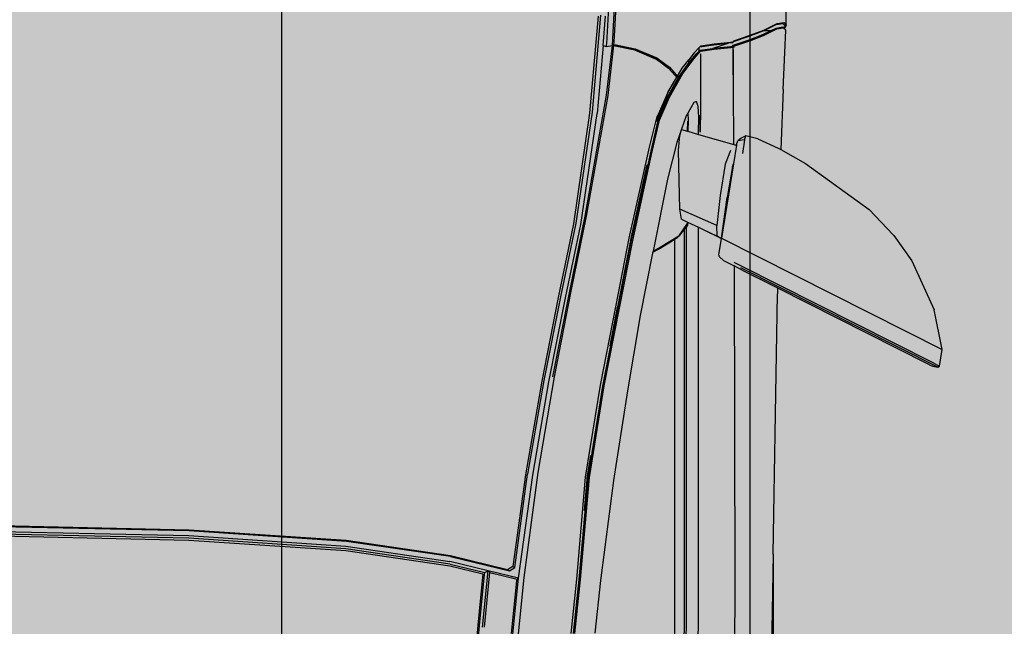
# Model space of a CAD drawing. Units: inches. Extents: x 1884 to 2398, y 474 to 1488.
# Tile 13 of 39: x 2231 to 2275, y 672 to 699. Entities that reach past the tile are written whole.
import ezdxf

# ---------------------------------------------------------------- set-up
doc = ezdxf.new("R2010")
doc.units = ezdxf.units.IN
doc.header["$MEASUREMENT"] = 0
doc.layers.get('0').update_dxf_attribs({"color": 250})
doc.layers.add('A-ANNO-DIMS', color=2, linetype='Continuous', lineweight=18)
doc.layers.add('C-VEHI', color=8, linetype='Continuous', lineweight=18)
doc.layers.add('Edges', color=250, linetype='Continuous')
doc.layers.add('L-PVMT-PATT', color=9, linetype='Continuous', lineweight=13, true_color=0xc7c8ca)
doc.styles.get("Standard").update_dxf_attribs({"font": 'arial.ttf'})
doc.dimstyles.get("Standard").update_dxf_attribs({"dimtxt": 7, "dimasz": 0.18, "dimexe": 0.18, "dimexo": 0.0625, "dimgap": 0.09, "dimtad": 0, "dimtih": 1, "dimtoh": 1, "dimzin": 0, "dimdsep": 46, "dimlunit": 3, "dimtxsty": 'Standard', "dimcen": 0.09, "dimadec": 0, "dimazin": 0, "dimtfac": 1, "dimtofl": 0, "dimtmove": 0, "dimatfit": 3, "dimfxl": 1, "dimtolj": 1, "dimtzin": 0, "dimarcsym": 0})

# ---------------------------------------------------------------- blocks, each defined once
blk = doc.blocks.new('Nissan Qashqai pl')
at = {"layer": 'Edges'}
for p, q in [((8.8918, 12.7444), (9.0186, 12.9956)), ((9.0386, 12.9907), (8.9254, 12.7664)), ((9.0186, 12.9956), (8.9731, 12.9865)), ((9.0374, 12.9925), (9.0186, 12.9956)), ((9.0356, 12.9888), (9.0374, 12.9925)), ((9.0386, 12.9907), (9.0374, 12.9925)), ((9.0376, 12.985), (9.0386, 12.9907)), ((8.9173, 12.961), (8.9731, 12.9865)), ((9.0333, 12.9845), (8.9232, 12.7662)), ((9.0356, 12.9888), (9.0333, 12.9845)), ((9.0343, 12.9785), (9.0347, 12.9794)), ((9.0347, 12.9794), (9.0362, 12.9822)), ((9.0362, 12.9822), (9.037, 12.9838)), ((9.0371, 12.9841), (9.037, 12.9838)), ((9.0371, 12.9841), (9.0376, 12.985)), ((9.0376, 12.985), (9.0371, 12.9847)), ((8.9483, 12.8082), (9.0343, 12.9785)), ((8.8885, 12.9405), (8.9173, 12.961)), ((8.8591, 12.9127), (8.8879, 12.94)), ((8.8885, 12.9405), (8.8879, 12.94)), ((8.8066, 12.84), (8.8591, 12.9127)), ((8.7908, 12.812), (8.8066, 12.84)), ((8.6489, 12.8179), (8.5719, 12.8193)), ((8.646, 12.8153), (8.6489, 12.8179)), ((8.646, 12.8153), (8.646, 12.8153)), ((8.6472, 12.8076), (8.646, 12.8153)), ((8.647, 12.8142), (8.6498, 12.8168)), ((8.6482, 12.8067), (8.647, 12.8142)), ((8.6489, 12.8179), (8.6527, 12.8156)), ((8.6498, 12.8168), (8.6524, 12.8153)), ((8.651, 12.814), (8.652, 12.815)), ((8.6524, 12.8064), (8.651, 12.814)), ((8.652, 12.815), (8.6524, 12.8153)), ((8.6534, 12.8073), (8.652, 12.815)), ((8.6524, 12.8153), (8.6527, 12.8156)), ((8.6527, 12.8156), (8.6537, 12.8167)), ((8.6547, 12.8176), (8.6537, 12.8167)), ((8.6537, 12.8167), (8.6537, 12.8166)), ((8.7222, 12.8144), (8.6547, 12.8176)), ((8.7222, 12.8144), (8.7908, 12.812)), ((8.7891, 12.8089), (8.7908, 12.812)), ((8.6546, 12.7926), (8.6472, 12.8076)), ((8.655, 12.7929), (8.6482, 12.8067)), ((8.655, 12.801), (8.6524, 12.8064)), ((8.6608, 12.7921), (8.6534, 12.8073)), ((8.6598, 12.7913), (8.655, 12.801)), ((8.655, 12.7929), (8.655, 12.801)), ((8.7785, 12.7855), (8.7891, 12.8089)), ((8.928, 12.7679), (8.9483, 12.8082)), ((8.9483, 12.8082), (8.9552, 12.8081)), ((9.2517, 12.8031), (8.9552, 12.8081)), ((9.2517, 12.8031), (9.351, 12.803)), ((9.2517, 12.8031), (9.5372, 12.7983)), ((8.6606, 12.7768), (8.6546, 12.7926)), ((8.6556, 12.7918), (8.655, 12.7929)), ((8.655, 12.7922), (8.655, 12.7929)), ((8.6616, 12.7758), (8.6556, 12.7918)), ((8.6657, 12.7758), (8.6598, 12.7913)), ((8.6667, 12.7767), (8.6608, 12.7921)), ((8.7785, 12.7855), (8.7751, 12.7719)), ((8.6667, 12.7584), (8.6606, 12.7768)), ((8.6675, 12.758), (8.6616, 12.7758)), ((8.6718, 12.7574), (8.6657, 12.7758)), ((8.6728, 12.7584), (8.6667, 12.7767)), ((8.7751, 12.7719), (8.7779, 12.7668)), ((8.7798, 12.7703), (8.7751, 12.7719)), ((8.7779, 12.7668), (8.7807, 12.763)), ((8.7798, 12.7703), (8.7807, 12.763)), ((8.7798, 12.7703), (8.7954, 12.7683)), ((8.9232, 12.7662), (8.9194, 12.7588)), ((8.928, 12.7679), (8.925, 12.762)), ((8.6675, 12.758), (8.6667, 12.7584)), ((8.6679, 12.7578), (8.6675, 12.758)), ((8.6676, 12.7576), (8.6675, 12.7576)), ((8.6675, 12.7576), (8.6675, 12.7576)), ((8.6675, 12.7576), (8.6676, 12.7576)), ((8.6676, 12.7576), (8.6677, 12.7576)), ((8.6677, 12.7576), (8.6677, 12.7576)), ((8.6677, 12.7576), (8.6682, 12.7576)), ((8.6682, 12.7576), (8.6679, 12.7578)), ((8.6682, 12.7576), (8.6692, 12.7566)), ((8.6682, 12.7572), (8.6682, 12.7576)), ((8.6684, 12.7554), (8.6682, 12.7572)), ((8.6682, 12.7572), (8.6692, 12.7566)), ((8.6684, 12.7554), (8.6685, 12.7549)), ((8.6684, 12.755), (8.6684, 12.7554)), ((8.6703, 12.7361), (8.6684, 12.755)), ((8.6692, 12.7566), (8.6697, 12.7519)), ((8.6729, 12.7568), (8.6718, 12.7574)), ((8.674, 12.7578), (8.6728, 12.7584)), ((8.6733, 12.7566), (8.6729, 12.7568)), ((8.6735, 12.7544), (8.6733, 12.7566)), ((8.6742, 12.7576), (8.674, 12.7578)), ((8.6742, 12.7584), (8.6743, 12.7582)), ((8.6744, 12.755), (8.6742, 12.7576)), ((8.6744, 12.7576), (8.6742, 12.7576)), ((8.6744, 12.7578), (8.6744, 12.7576)), ((8.6773, 12.7577), (8.6744, 12.7576)), ((8.6764, 12.736), (8.6744, 12.755)), ((8.6791, 12.7578), (8.677, 12.7578)), ((8.6791, 12.7577), (8.6773, 12.7577)), ((8.7205, 12.7579), (8.6791, 12.7578)), ((8.6791, 12.7577), (8.6791, 12.7578)), ((8.6878, 12.7577), (8.6791, 12.7578)), ((8.6878, 12.7577), (8.6791, 12.7577)), ((8.6878, 12.7577), (8.6878, 12.7577)), ((8.6911, 12.7577), (8.6878, 12.7577)), ((8.7205, 12.7579), (8.6911, 12.7577)), ((8.7849, 12.7582), (8.7205, 12.7579)), ((8.7734, 12.7181), (8.7849, 12.7582)), ((8.7849, 12.7615), (8.7807, 12.763)), ((8.7849, 12.7615), (8.7858, 12.7613)), ((8.7849, 12.7582), (8.7856, 12.7608)), ((8.7858, 12.7613), (8.7856, 12.7608)), ((8.7858, 12.7613), (8.807, 12.758)), ((8.8102, 12.7568), (8.807, 12.758)), ((8.807, 12.758), (8.8918, 12.7444)), ((8.8102, 12.7568), (8.8455, 12.7506)), ((8.9171, 12.7464), (8.9233, 12.7586)), ((8.925, 12.762), (8.9233, 12.7586)), ((8.9233, 12.7586), (9.2886, 12.7594)), ((9.2886, 12.7594), (9.4673, 12.7589)), ((8.6697, 12.7519), (8.6698, 12.7516)), ((8.6714, 12.7353), (8.6697, 12.7519)), ((8.6698, 12.7516), (8.6755, 12.7343)), ((8.6754, 12.7353), (8.6735, 12.7544)), ((8.7917, 12.7547), (8.8075, 12.7486)), ((8.8075, 12.7486), (8.8429, 12.7426)), ((8.8918, 12.7444), (8.8455, 12.7506)), ((8.8815, 12.7228), (8.892, 12.7444)), ((8.892, 12.7444), (8.8908, 12.7421)), ((8.8911, 12.7428), (8.8919, 12.7444)), ((8.8911, 12.7428), (8.8919, 12.7444)), ((8.8919, 12.7444), (8.8911, 12.7428)), ((8.8919, 12.7444), (8.8918, 12.7444)), ((8.892, 12.7444), (8.8919, 12.7444)), ((8.8919, 12.7444), (8.8919, 12.7444)), ((8.8919, 12.7444), (8.8919, 12.7444)), ((8.9106, 12.7413), (8.892, 12.7444)), ((8.892, 12.7444), (8.892, 12.7444)), ((8.9171, 12.7464), (8.9131, 12.7421)), ((8.9171, 12.7464), (8.917, 12.7468)), ((8.6727, 12.7207), (8.6703, 12.7361)), ((8.6737, 12.7197), (8.6714, 12.7353)), ((8.6755, 12.7343), (8.6754, 12.7353)), ((8.6777, 12.7196), (8.6755, 12.7343)), ((8.6764, 12.7359), (8.6764, 12.736)), ((8.6788, 12.7205), (8.6764, 12.7359)), ((8.8429, 12.7426), (8.8771, 12.7388)), ((8.8771, 12.7388), (8.8585, 12.6969)), ((8.8895, 12.7393), (8.8771, 12.7388)), ((8.8815, 12.7228), (8.8895, 12.7393)), ((8.8908, 12.7421), (8.8895, 12.7393)), ((8.8906, 12.7418), (8.8895, 12.7393)), ((8.8906, 12.7418), (8.8911, 12.7428)), ((8.9131, 12.7421), (8.9106, 12.7413)), ((8.8793, 12.7181), (8.8815, 12.7228)), ((8.6737, 12.7197), (8.6727, 12.7207)), ((8.6746, 12.7189), (8.6737, 12.7197)), ((8.6785, 12.7189), (8.6746, 12.7189)), ((8.6805, 12.7132), (8.6746, 12.7189)), ((8.6785, 12.7189), (8.6777, 12.7196)), ((8.6815, 12.7162), (8.6785, 12.7189)), ((8.687, 12.7132), (8.6788, 12.7205)), ((8.6805, 12.7132), (8.6884, 12.7071)), ((8.6815, 12.7162), (8.6818, 12.7154)), ((8.6817, 12.716), (8.6815, 12.7162)), ((8.6817, 12.716), (8.6818, 12.7154)), ((8.6859, 12.7122), (8.6817, 12.716)), ((8.6818, 12.7204), (8.7012, 12.7203)), ((8.6818, 12.7154), (8.6902, 12.7081)), ((8.6927, 12.7071), (8.6859, 12.7122)), ((8.7042, 12.7002), (8.687, 12.7132)), ((8.7012, 12.7203), (8.7012, 12.7203)), ((8.7012, 12.7203), (8.7026, 12.7203)), ((8.7026, 12.7203), (8.7026, 12.7203)), ((8.7026, 12.7203), (8.7072, 12.7203)), ((8.7072, 12.7203), (8.7072, 12.7203)), ((8.7072, 12.7203), (8.7273, 12.7202)), ((8.7273, 12.7202), (8.7273, 12.7201)), ((8.7273, 12.7202), (8.7354, 12.7202)), ((8.7354, 12.7201), (8.7354, 12.7202)), ((8.7354, 12.7202), (8.742, 12.7202)), ((8.7415, 12.7177), (8.7361, 12.7158)), ((8.7361, 12.7158), (8.7373, 12.7128)), ((8.7373, 12.7128), (8.7492, 12.7059)), ((8.7534, 12.7185), (8.7415, 12.7177)), ((8.742, 12.7201), (8.742, 12.7202)), ((8.742, 12.7202), (8.742, 12.7201)), ((8.742, 12.7202), (8.742, 12.7202)), ((8.742, 12.7202), (8.7426, 12.7202)), ((8.7426, 12.7201), (8.7426, 12.7202)), ((8.7426, 12.7202), (8.7433, 12.7202)), ((8.7433, 12.7201), (8.7433, 12.7202)), ((8.7433, 12.7202), (8.7711, 12.7201)), ((8.7711, 12.7201), (8.7516, 12.72)), ((8.7718, 12.7181), (8.7534, 12.7185)), ((8.7698, 12.7058), (8.7734, 12.7181)), ((8.7734, 12.7181), (8.7718, 12.7181)), ((8.8734, 12.7057), (8.8793, 12.7181)), ((9.3194, 12.7179), (8.8793, 12.7181)), ((9.4919, 12.7173), (9.3194, 12.7179)), ((8.6917, 12.7071), (8.6884, 12.7071)), ((8.698, 12.6996), (8.6884, 12.7071)), ((8.6902, 12.7081), (8.6917, 12.7071)), ((8.6917, 12.7071), (8.7075, 12.6955)), ((8.6927, 12.7071), (8.6923, 12.7071)), ((8.7032, 12.6992), (8.6927, 12.7071)), ((8.7071, 12.6942), (8.698, 12.6996)), ((8.7302, 12.684), (8.7032, 12.6992)), ((8.7312, 12.6851), (8.7042, 12.7002)), ((8.7492, 12.7059), (8.7572, 12.7062)), ((8.7492, 12.7059), (8.7524, 12.704)), ((8.7524, 12.704), (8.7828, 12.6934)), ((8.7572, 12.7062), (8.7698, 12.7058)), ((8.7698, 12.7057), (8.7583, 12.706)), ((8.7678, 12.6988), (8.7698, 12.7057)), ((8.7748, 12.6967), (8.7678, 12.6988)), ((8.7698, 12.7057), (8.7698, 12.7058)), ((8.87, 12.6987), (8.8734, 12.7057)), ((8.8734, 12.7057), (8.8768, 12.7057)), ((8.8751, 12.7054), (8.8768, 12.7057)), ((8.8893, 12.6956), (8.8751, 12.7054)), ((8.8768, 12.7057), (8.879, 12.704)), ((8.879, 12.704), (9.3198, 12.7039)), ((8.879, 12.704), (8.881, 12.7023)), ((9.3225, 12.7021), (8.881, 12.7023)), ((8.881, 12.7023), (8.8893, 12.6956)), ((9.3198, 12.7039), (9.4922, 12.7033)), ((9.4936, 12.7013), (9.3225, 12.7021)), ((8.697, 12.685), (8.7055, 12.6927)), ((8.6979, 12.6839), (8.7062, 12.6915)), ((8.7062, 12.6915), (8.6987, 12.6845)), ((8.7055, 12.6927), (8.7071, 12.6942)), ((8.7062, 12.6915), (8.7067, 12.6919)), ((8.7067, 12.6919), (8.7083, 12.6934)), ((8.7071, 12.6942), (8.7083, 12.6934)), ((8.7075, 12.6955), (8.7346, 12.6806)), ((8.7083, 12.6934), (8.7083, 12.6934)), ((8.7083, 12.6934), (8.7083, 12.6934)), ((8.7102, 12.6923), (8.7083, 12.6934)), ((8.7083, 12.6934), (8.7083, 12.6934)), ((8.7108, 12.6919), (8.7102, 12.6923)), ((8.7102, 12.6923), (8.7102, 12.6923)), ((8.7257, 12.6833), (8.7108, 12.6919)), ((8.7248, 12.6836), (8.7108, 12.6919)), ((8.7916, 12.6954), (8.7748, 12.6967)), ((8.7828, 12.6934), (8.8245, 12.6828)), ((8.8259, 12.6959), (8.7916, 12.6954)), ((8.8585, 12.6969), (8.8259, 12.6959)), ((8.87, 12.6987), (8.8585, 12.6969)), ((8.8893, 12.6956), (8.9021, 12.6745)), ((8.8913, 12.6936), (8.8893, 12.6956)), ((8.8927, 12.6913), (8.8913, 12.6936)), ((9.3224, 12.6911), (8.8927, 12.6913)), ((8.9041, 12.6725), (8.8927, 12.6913)), ((9.3225, 12.6911), (9.3224, 12.6911)), ((9.4936, 12.6904), (9.3225, 12.6911)), ((8.6864, 12.6706), (8.697, 12.685)), ((8.6875, 12.6698), (8.6979, 12.6839)), ((8.6987, 12.6845), (8.6924, 12.676)), ((8.7257, 12.6833), (8.7248, 12.6836)), ((8.7257, 12.6832), (8.7257, 12.6833)), ((8.7257, 12.6832), (8.7508, 12.672)), ((8.7529, 12.6741), (8.7302, 12.684)), ((8.7574, 12.6737), (8.7312, 12.6851)), ((8.7346, 12.6806), (8.7491, 12.6738)), ((8.7346, 12.6806), (8.7577, 12.6709)), ((8.8245, 12.6828), (8.9063, 12.6663)), ((8.6759, 12.6459), (8.6864, 12.6706)), ((8.6772, 12.6454), (8.6875, 12.6698)), ((8.6883, 12.6704), (8.6777, 12.6457)), ((8.6924, 12.676), (8.6883, 12.6704)), ((8.6924, 12.676), (8.6924, 12.6762)), ((8.7508, 12.672), (8.7491, 12.6738)), ((8.7491, 12.6738), (8.7576, 12.6699)), ((8.7532, 12.6708), (8.7508, 12.672)), ((8.7529, 12.6741), (8.7577, 12.6709)), ((8.757, 12.6724), (8.7529, 12.6741)), ((8.7575, 12.6698), (8.7532, 12.6708)), ((8.7587, 12.672), (8.757, 12.6724)), ((8.7931, 12.6653), (8.7574, 12.6737)), ((8.7576, 12.6699), (8.7575, 12.6698)), ((8.7881, 12.6621), (8.7575, 12.6698)), ((8.7582, 12.6707), (8.7576, 12.6699)), ((8.7577, 12.6709), (8.7582, 12.6707)), ((8.759, 12.6717), (8.7582, 12.6707)), ((8.7587, 12.672), (8.759, 12.6717)), ((8.7591, 12.6719), (8.7587, 12.672)), ((8.7591, 12.6719), (8.759, 12.6717)), ((8.7925, 12.664), (8.7591, 12.6719)), ((8.8942, 12.6432), (8.7931, 12.6653)), ((8.9021, 12.6745), (8.9063, 12.6663)), ((8.9075, 12.6661), (8.9041, 12.6725)), ((8.9063, 12.6663), (8.9075, 12.6661)), ((8.9075, 12.6661), (8.9087, 12.6658)), ((8.9087, 12.6658), (8.9797, 12.6518)), ((8.8918, 12.6392), (8.7881, 12.6621)), ((8.8941, 12.6418), (8.7925, 12.664)), ((8.8083, 12.6591), (8.8954, 12.6403)), ((8.6716, 12.6242), (8.6759, 12.6459)), ((8.6772, 12.6454), (8.6721, 12.6201)), ((8.6777, 12.6457), (8.6727, 12.6213)), ((8.9696, 12.6285), (8.8942, 12.6432)), ((8.9797, 12.6518), (9.0656, 12.6372)), ((8.9679, 12.6241), (8.8918, 12.6392)), ((9.0601, 12.6092), (8.8941, 12.6418)), ((8.8961, 12.6401), (8.9704, 12.6257)), ((9.0656, 12.6372), (9.1676, 12.6212)), ((8.6197, 12.6241), (8.6683, 12.6215)), ((8.6721, 12.6201), (8.6204, 12.6229)), ((8.6683, 12.6215), (8.671, 12.6214)), ((8.671, 12.6214), (8.6716, 12.6242)), ((8.671, 12.6214), (8.6721, 12.6201)), ((8.6727, 12.6213), (8.6721, 12.6201)), ((8.6727, 12.6213), (8.6753, 12.621)), ((8.6753, 12.621), (8.7292, 12.6146)), ((9.0591, 12.6065), (8.9679, 12.6241)), ((9.06, 12.6106), (8.9696, 12.6285)), ((8.9704, 12.6257), (8.9708, 12.6256)), ((8.9708, 12.6256), (9.0143, 12.6169)), ((9.1676, 12.6212), (9.2814, 12.6065)), ((8.622, 12.6161), (8.6699, 12.6132)), ((8.6721, 12.6093), (8.6387, 12.6123)), ((8.6699, 12.6132), (8.6721, 12.613)), ((8.6733, 12.6129), (8.6721, 12.6201)), ((8.7287, 12.6134), (8.6721, 12.6201)), ((8.6721, 12.6127), (8.6721, 12.613)), ((8.6721, 12.613), (8.6733, 12.6129)), ((8.6721, 12.6093), (8.6733, 12.6129)), ((8.6721, 12.6093), (8.7496, 12.6025)), ((8.8666, 12.5888), (8.7287, 12.6134)), ((8.7292, 12.6146), (8.8666, 12.5901)), ((9.1644, 12.5938), (9.06, 12.6106)), ((9.1645, 12.5924), (9.0601, 12.6092)), ((8.6375, 12.6066), (8.7481, 12.5968)), ((8.6386, 12.6037), (8.7491, 12.594)), ((8.8761, 12.5839), (8.7496, 12.6025)), ((9.1639, 12.5895), (9.0591, 12.6065)), ((9.2814, 12.6065), (9.3416, 12.5999)), ((8.7481, 12.5968), (8.8745, 12.5782)), ((8.7491, 12.594), (8.8754, 12.5755)), ((8.8666, 12.5901), (8.9521, 12.5726)), ((8.9522, 12.5713), (8.8666, 12.5888)), ((9.1393, 12.5951), (9.1647, 12.591)), ((9.2801, 12.5794), (9.1639, 12.5895)), ((9.2803, 12.5836), (9.1644, 12.5938)), ((9.2804, 12.5821), (9.1645, 12.5924)), ((9.1647, 12.591), (9.1668, 12.5908)), ((9.1668, 12.5908), (9.2019, 12.5877)), ((8.8745, 12.5782), (8.9583, 12.5609)), ((8.8754, 12.5755), (8.9591, 12.5583)), ((8.9598, 12.5666), (8.8761, 12.5839)), ((9.3418, 12.5729), (9.2801, 12.5794)), ((9.3418, 12.5771), (9.2803, 12.5836)), ((9.3419, 12.5756), (9.2804, 12.5821)), ((8.9521, 12.5726), (9.0495, 12.5536)), ((9.0497, 12.5523), (8.9522, 12.5713)), ((9.0552, 12.5477), (8.9598, 12.5666)), ((8.9583, 12.5609), (9.0538, 12.5419)), ((8.9591, 12.5583), (9.0546, 12.5394)), ((9.0495, 12.5536), (9.1584, 12.5351)), ((9.0538, 12.5419), (9.1605, 12.5233)), ((9.1617, 12.5292), (9.0552, 12.5477)), ((9.0546, 12.5394), (9.1612, 12.5208)), ((9.1584, 12.5351), (9.2783, 12.5191)), ((9.2669, 12.5088), (9.1605, 12.5233)), ((9.1612, 12.5208), (9.2656, 12.5065)), ((9.2789, 12.5131), (9.1617, 12.5292)), ((9.2656, 12.5065), (9.2669, 12.5088)), ((9.2707, 12.5028), (9.2669, 12.5088)), ((9.2789, 12.5131), (9.2704, 12.4783)), ((9.2724, 12.4804), (9.2799, 12.5114)), ((9.2783, 12.5191), (9.3422, 12.5126)), ((9.2799, 12.5114), (9.2789, 12.5131)), ((9.3427, 12.5066), (9.2789, 12.5131)), ((9.2819, 12.5112), (9.2799, 12.5114)), ((9.2803, 12.5116), (9.2822, 12.5118)), ((9.3418, 12.5051), (9.2819, 12.5112)), ((9.2694, 12.5006), (9.2535, 12.4354)), ((9.2543, 12.4356), (9.2707, 12.5028)), ((9.2656, 12.5065), (9.2694, 12.5006)), ((9.2707, 12.5028), (9.2694, 12.5006)), ((9.2704, 12.4783), (9.2598, 12.4348)), ((9.2629, 12.435), (9.2726, 12.4746)), ((9.2724, 12.4804), (9.2704, 12.4783)), ((9.2726, 12.4746), (9.2704, 12.4783)), ((9.3346, 12.4718), (9.2704, 12.4783)), ((9.3346, 12.4741), (9.2724, 12.4804)), ((9.2746, 12.4744), (9.2726, 12.4746)), ((9.2649, 12.4348), (9.2741, 12.4725)), ((9.2741, 12.4725), (9.3326, 12.4666)), ((9.333, 12.4685), (9.2746, 12.4744)), ((9.3326, 12.4666), (9.4, 12.4609)), ((9.4004, 12.4629), (9.333, 12.4685)), ((9.2535, 12.4354), (9.2362, 12.3167)), ((9.2543, 12.4356), (9.2371, 12.3169)), ((9.2426, 12.3164), (9.2598, 12.4348)), ((9.2629, 12.435), (9.2457, 12.3164)), ((9.2476, 12.3163), (9.2649, 12.4348)), ((9.2362, 12.3167), (9.2241, 12.1376)), ((9.2371, 12.3169), (9.2249, 12.1376)), ((9.2305, 12.1375), (9.2426, 12.3164)), ((9.2457, 12.3164), (9.2335, 12.1374)), ((9.2355, 12.1374), (9.2476, 12.3163)), ((9.2241, 12.1376), (9.2195, 11.9221)), ((9.2249, 12.1376), (9.2203, 11.9221)), ((9.2259, 11.9221), (9.2305, 12.1375)), ((9.2335, 12.1374), (9.2289, 11.9221)), ((9.2308, 11.9221), (9.2355, 12.1374))]:
    blk.add_line(p, q, dxfattribs=at)
blk = doc.blocks.new('car')
blk.add_blockref('Nissan Qashqai pl', (-9.7433, -11.9151))
blk = doc.blocks.new('carr')
blk.add_blockref('car', (0.5124, -0.007))
blk = doc.blocks.new('*D23')
at = {"layer": 'A-ANNO-DIMS', "color": 0, "lineweight": -2, "transparency": 16777216}
for p, q in [((2272.304, 752.812), (2298.291, 752.812)), ((2298.111, 752.632), (2298.111, 670.29)), ((2298.111, 580.529), (2298.111, 662.871)), ((2272.304, 580.349), (2298.291, 580.349))]:
    blk.add_line(p, q, dxfattribs=at)
at = {"layer": 'A-ANNO-DIMS', "color": 0, "lineweight": 100, "transparency": 16777216}
for points in [[(2298.081, 752.632), (2298.141, 752.632), (2298.111, 752.812)], [(2298.081, 580.529), (2298.141, 580.529), (2298.111, 580.349)]]:
    blk.add_solid(points, dxfattribs=at)
at = {"layer": 'Defpoints', "color": 0, "lineweight": 100, "transparency": 16777216}
for p in [(2272.242, 752.812), (2272.242, 580.349), (2298.111, 580.349)]:
    blk.add_point(p, dxfattribs=at)
at = {"layer": 'A-ANNO-DIMS', "color": 0, "transparency": 16777216, "insert": (2298.111, 666.58), "char_height": 7, "attachment_point": 5}
blk.add_mtext('\\A1;CAR 14\'-4 1/2" TYP.', dxfattribs=at)
blk = doc.blocks.new('*D44')
at = {"layer": 'A-ANNO-DIMS', "color": 0, "lineweight": -2, "transparency": 16777216}
for p, q in [((2209.755, 1247.822), (2209.755, 484.005)), ((2230.029, 1247.822), (2230.029, 484.005)), ((2209.935, 484.185), (2229.849, 484.185)), ((2230.029, 484.185), (2230.209, 484.185))]:
    blk.add_line(p, q, dxfattribs=at)
at = {"layer": 'A-ANNO-DIMS', "color": 0, "lineweight": 100, "transparency": 16777216}
for points in [[(2209.935, 484.215), (2209.935, 484.155), (2209.755, 484.185)], [(2229.849, 484.215), (2229.849, 484.155), (2230.029, 484.185)]]:
    blk.add_solid(points, dxfattribs=at)
at = {"layer": 'Defpoints', "color": 0, "lineweight": 100, "transparency": 16777216}
for p in [(2209.755, 1247.885), (2230.029, 1247.885), (2230.029, 484.185)]:
    blk.add_point(p, dxfattribs=at)
at = {"layer": 'A-ANNO-DIMS', "color": 0, "transparency": 16777216, "insert": (2247.429, 484.185), "char_height": 7, "attachment_point": 5}
blk.add_mtext('\\A1;1\'-8 1/2"', dxfattribs=at)
blk = doc.blocks.new('*D45')
at = {"layer": 'A-ANNO-DIMS', "color": 0, "lineweight": -2, "transparency": 16777216}
for p, q in [((2242.617, 1322.822), (2242.617, 484.005)), ((2263.617, 1322.822), (2263.617, 484.005)), ((2242.797, 484.185), (2244.052, 484.185)), ((2263.437, 484.185), (2262.181, 484.185))]:
    blk.add_line(p, q, dxfattribs=at)
at = {"layer": 'A-ANNO-DIMS', "color": 0, "lineweight": 100, "transparency": 16777216}
for points in [[(2242.797, 484.215), (2242.797, 484.155), (2242.617, 484.185)], [(2263.437, 484.215), (2263.437, 484.155), (2263.617, 484.185)]]:
    blk.add_solid(points, dxfattribs=at)
at = {"layer": 'Defpoints', "color": 0, "lineweight": 100, "transparency": 16777216}
for p in [(2242.617, 1322.885), (2263.617, 1322.885), (2263.617, 484.185)]:
    blk.add_point(p, dxfattribs=at)
at = {"layer": 'A-ANNO-DIMS', "color": 0, "transparency": 16777216, "insert": (2253.117, 484.185), "char_height": 7, "attachment_point": 5}
blk.add_mtext('\\A1;1\'-9"', dxfattribs=at)

msp = doc.modelspace()

# ---------------------------------------------------------------- hatches: boundary and pattern name
at = {"layer": 'L-PVMT-PATT'}
h = msp.add_hatch(color=256, dxfattribs=at)
h.dxf.hatch_style = 1
h.paths.add_polyline_path([(2387.529, 769.966), (2351.529, 769.966), (2238.447, 769.966), (2238.447, 762.15), (2238.447, 754.445), (2126.529, 754.445), (2126.529, 676.183), (2134.868, 676.183), (2142.673, 676.183), (2142.673, 646.578), (2134.868, 646.578), (2126.529, 646.578), (2126.529, 640.17), (2387.529, 640.17)])
h.paths.add_polyline_path([(2387.529, 631.385), (2303.086, 631.385), (2303.086, 615.671), (2387.529, 615.671)])
h.paths.add_polyline_path([(2387.529, 640.17), (2126.529, 640.17), (2126.529, 631.385), (2387.529, 631.385)])
h.paths.add_polyline_path([(2393.529, 604.13), (2387.529, 604.13), (2387.529, 615.671), (2303.086, 615.671), (2303.086, 607.943), (2249.649, 607.943), (2126.529, 607.943), (2126.529, 533.885), (2393.529, 533.885)])
h.paths.add_polyline_path([(2257.825, 611.008), (2257.83, 611.337), (2257.915, 616.493), (2258.021, 621.805), (2258.146, 627.274), (2258.252, 631.385), (2126.529, 631.385), (2126.529, 611.008)])
h.paths.add_polyline_path([(2258.892, 611.285), (2258.888, 611.008), (2300.247, 611.008), (2300.247, 631.385), (2259.314, 631.385), (2259.206, 627.173), (2259.081, 621.72), (2258.976, 616.424)])

# ---------------------------------------------------------------- block references
at = {"layer": 'C-VEHI', "xscale": 39.37007874015748, "yscale": 39.37007874015748, "zscale": 39.37007874015748, "rotation": 270}
msp.add_blockref('carr', (2229.977, 676.232), dxfattribs=at)

# ---------------------------------------------------------------- dimensions: what is measured, and where the dimension line sits
at = {"layer": 'A-ANNO-DIMS'}
for base, p1, p2, picture, middle in [((2263.617, 484.185), (2242.617, 1322.885), (2263.617, 1322.885), '*D45', (2253.117, 484.185)), ((2230.029, 484.185), (2209.755, 1247.885), (2230.029, 1247.885), '*D44', (2247.429, 484.185))]:
    dim = msp.add_linear_dim(base=base, p1=p1, p2=p2, dimstyle='Standard', override={"dimdec": 1, "dimlfac": 1, "dimrnd": 0, "dimzin": 1, "dimdsep": 46, "dimlunit": 4, "dimfrac": 2}, dxfattribs=at)
    dim.commit()
    dim.dimension.update_dxf_attribs({"geometry": picture, "text_midpoint": middle})
dim = msp.add_linear_dim(base=(2298.111, 580.349), p1=(2272.242, 752.812), p2=(2272.242, 580.349), angle=270, text='CAR <> TYP.', dimstyle='Standard', override={"dimdec": 1, "dimlfac": 1, "dimrnd": 0, "dimzin": 1, "dimdsep": 46, "dimlunit": 4, "dimfrac": 2}, dxfattribs=at)
dim.commit()
dim.dimension.update_dxf_attribs({"geometry": '*D23', "text_midpoint": (2298.111, 666.58)})

doc.saveas('drawing.dxf')
